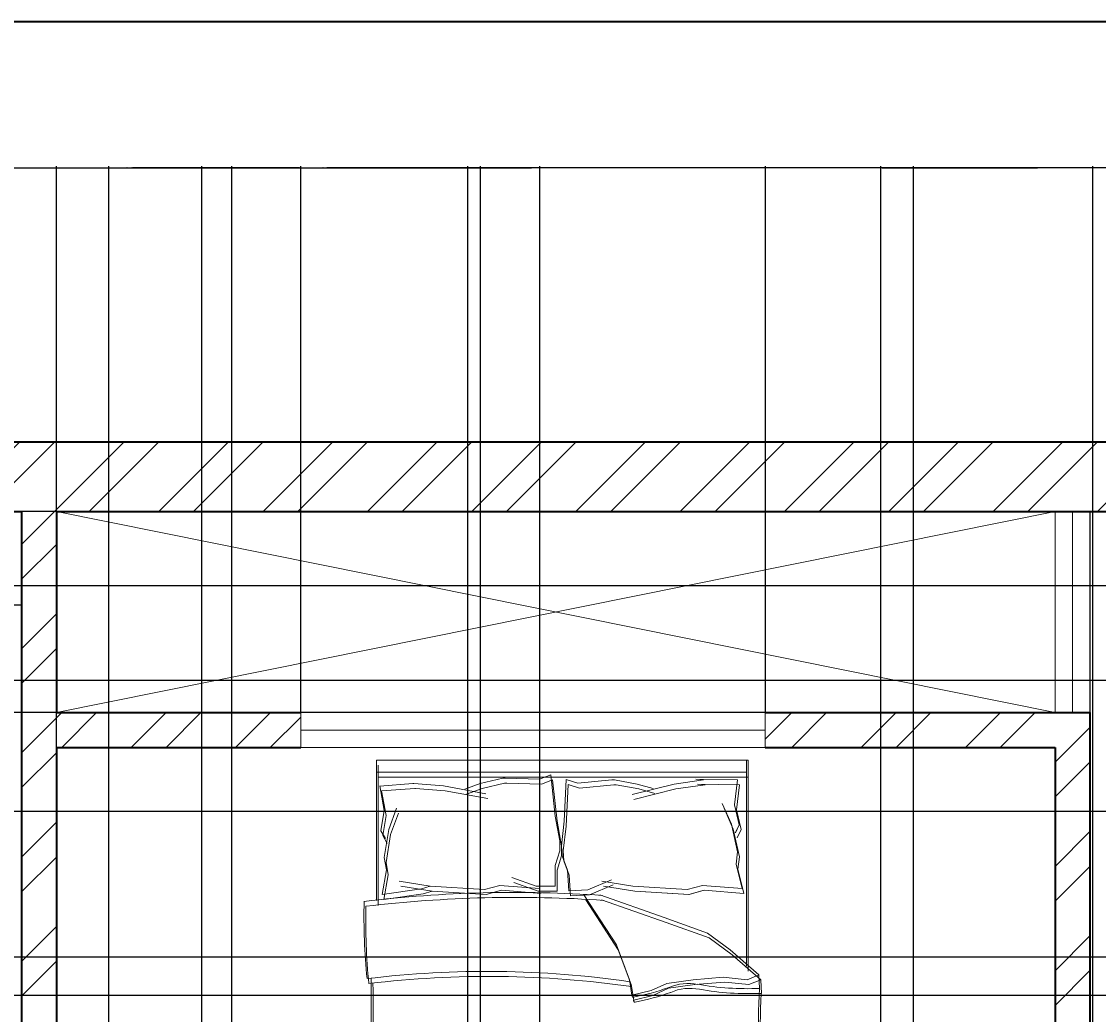
# Model space of a CAD drawing. Units: inches. Extents: x 2529 to 3014, y 1203 to 2262.
# Tile 12 of 13: x 2733 to 2872, y 2133 to 2262. Entities that reach past the tile are written whole.
import ezdxf

# ---------------------------------------------------------------- set-up
doc = ezdxf.new("R2010")
doc.units = ezdxf.units.IN
for name, color, linetype, lineweight in [('A-ANNO-DIMS', 2, 'Continuous', 18), ('A-ANNO-TTLB', 7, 'Continuous', 35), ('A-FLOR-CASE', 7, 'Continuous', 25), ('A-FLOR-OPEN', 61, 'Continuous', 13), ('A-FURN', 8, 'Continuous', 18), ('A-GLAZ', 191, 'Continuous', 18), ('A-WALL', 7, 'Continuous', 35), ('A-WALL-PATT', 143, 'Continuous', 13)]:
    doc.layers.add(name, color=color, linetype=linetype, lineweight=lineweight)
doc.styles.get("Standard").update_dxf_attribs({"font": 'arial.ttf'})
doc.dimstyles.get("Standard").update_dxf_attribs({"dimtxt": 0.18, "dimasz": 0.18, "dimexe": 0.18, "dimexo": 0.0625, "dimgap": 0.09, "dimtad": 0, "dimtih": 1, "dimtoh": 1, "dimdec": 4, "dimzin": 0, "dimdsep": 46, "dimtxsty": 'Standard', "dimcen": 0.09, "dimadec": 0, "dimazin": 0, "dimtfac": 1, "dimtdec": 4, "dimtofl": 0, "dimtmove": 0, "dimatfit": 3, "dimfxl": 1, "dimtolj": 1, "dimtzin": 0, "dimarcsym": 0})

# ---------------------------------------------------------------- blocks, each defined once
blk = doc.blocks.new('BED-DOUBLE')
for p, q in [((3.48, 63.33), (3.48, 81.44)), ((3.48, 63.33), (3.48, 81.44)), ((3.48, 81.44), (51.49, 81.44)), ((3.7, 62.69), (3.7, 80.8)), ((3.7, 62.69), (3.7, 80.8)), ((51.27, 81.44), (51.27, 54.83)), ((51.27, 81.44), (51.27, 54.83)), ((51.49, 81.44), (51.49, 80.8)), ((51.49, 80.8), (51.49, 54.19)), ((51.49, 80.8), (51.49, 54.19)), ((3.48, 79.91), (51.27, 79.91)), ((3.48, 79.91), (51.27, 79.91)), ((24.54, 78.99), (25.98, 79.57)), ((24.54, 78.99), (25.98, 79.57)), ((25.98, 79.57), (26.56, 74.22)), ((25.98, 79.57), (26.56, 74.22)), ((3.7, 79.27), (51.49, 79.27)), ((3.7, 79.27), (51.49, 79.27)), ((3.9, 78.11), (8.18, 78.43)), ((3.9, 78.11), (8.18, 78.43)), ((3.9, 78.13), (4.47, 74.95)), ((3.9, 78.13), (4.47, 74.95)), ((8.18, 78.43), (8.29, 78.42)), ((8.18, 78.43), (8.29, 78.42)), ((8.29, 78.42), (12.11, 78.13)), ((8.29, 78.42), (12.11, 78.13)), ((12.11, 78.13), (17.6, 77.12)), ((12.11, 78.13), (17.6, 77.12)), ((14.86, 77.69), (16.88, 78.42)), ((14.86, 77.69), (16.88, 78.42)), ((16.88, 78.42), (19.77, 79.14)), ((16.88, 78.42), (19.77, 79.14)), ((17.11, 77.78), (20, 78.5)), ((17.11, 77.78), (20, 78.5)), ((19.77, 79.14), (20.09, 79.14)), ((19.77, 79.14), (20.09, 79.14)), ((20, 78.5), (20.32, 78.5)), ((20, 78.5), (20.32, 78.5)), ((20.09, 79.14), (24.54, 78.99)), ((20.09, 79.14), (24.54, 78.99)), ((20.32, 78.5), (24.77, 78.36)), ((20.32, 78.5), (24.77, 78.36)), ((24.77, 78.36), (26.21, 78.93)), ((24.77, 78.36), (26.21, 78.93)), ((26.21, 78.93), (26.79, 73.58)), ((26.21, 78.93), (26.79, 73.58)), ((27.98, 78.95), (27.73, 73.58)), ((27.98, 78.95), (27.73, 73.58)), ((28.21, 78.31), (27.96, 72.94)), ((28.21, 78.31), (27.96, 72.94)), ((29.46, 78.46), (27.98, 78.95)), ((29.46, 78.46), (27.98, 78.95)), ((29.68, 77.83), (28.21, 78.31)), ((29.68, 77.83), (28.21, 78.31)), ((33.88, 78.89), (29.46, 78.46)), ((33.88, 78.89), (29.46, 78.46)), ((34.11, 78.25), (29.68, 77.83)), ((34.11, 78.25), (29.68, 77.83)), ((34.21, 78.91), (33.88, 78.89)), ((34.21, 78.91), (33.88, 78.89)), ((34.43, 78.27), (34.11, 78.25)), ((34.43, 78.27), (34.11, 78.25)), ((37.14, 78.37), (34.21, 78.91)), ((37.14, 78.37), (34.21, 78.91)), ((37.36, 77.73), (34.43, 78.27)), ((37.36, 77.73), (34.43, 78.27)), ((41.91, 78.37), (36.5, 77.02)), ((41.91, 78.37), (36.5, 77.02)), ((39.2, 77.77), (37.14, 78.37)), ((39.2, 77.77), (37.14, 78.37)), ((45.71, 78.9), (41.91, 78.37)), ((45.71, 78.9), (41.91, 78.37)), ((45.94, 78.26), (42.14, 77.73)), ((45.94, 78.26), (42.14, 77.73)), ((50.11, 78.89), (44.71, 78.98)), ((44.71, 78.98), (45.71, 78.9)), ((50.11, 78.89), (44.71, 78.98)), ((44.71, 78.98), (45.71, 78.9)), ((50.34, 78.25), (44.94, 78.34)), ((44.94, 78.34), (45.94, 78.26)), ((50.34, 78.25), (44.94, 78.34)), ((44.94, 78.34), (45.94, 78.26)), ((50.11, 78.89), (49.73, 75.68)), ((50.11, 78.89), (49.73, 75.68)), ((50.34, 78.25), (49.96, 75.04)), ((50.34, 78.25), (49.96, 75.04)), ((4.12, 77.49), (4.7, 74.31)), ((4.12, 77.49), (4.7, 74.31)), ((4.13, 77.47), (8.41, 77.8)), ((4.13, 77.47), (8.41, 77.8)), ((8.41, 77.8), (8.51, 77.78)), ((8.41, 77.8), (8.51, 77.78)), ((8.51, 77.78), (12.34, 77.49)), ((8.51, 77.78), (12.34, 77.49)), ((12.34, 77.49), (17.83, 76.48)), ((12.34, 77.49), (17.83, 76.48)), ((15.08, 77.05), (17.11, 77.78)), ((15.08, 77.05), (17.11, 77.78)), ((42.14, 77.73), (36.72, 76.38)), ((42.14, 77.73), (36.72, 76.38)), ((39.43, 77.13), (37.36, 77.73)), ((39.43, 77.13), (37.36, 77.73)), ((5.05, 72.49), (6.06, 75.24)), ((5.05, 72.49), (6.06, 75.24)), ((49.31, 73.19), (48.13, 75.87)), ((49.31, 73.19), (48.13, 75.87)), ((49.54, 72.55), (48.36, 75.23)), ((49.54, 72.55), (48.36, 75.23)), ((49.73, 75.68), (50.33, 73.11)), ((49.73, 75.68), (50.33, 73.11)), ((4.47, 74.95), (4.04, 72.34)), ((4.47, 74.95), (4.04, 72.34)), ((4.7, 74.31), (4.27, 71.7)), ((4.7, 74.31), (4.27, 71.7)), ((5.28, 71.85), (6.29, 74.6)), ((5.28, 71.85), (6.29, 74.6)), ((26.56, 74.22), (27.14, 71.04)), ((26.56, 74.22), (27.14, 71.04)), ((49.96, 75.04), (50.56, 72.47)), ((49.96, 75.04), (50.56, 72.47)), ((4.04, 72.34), (4.62, 71.33)), ((4.04, 72.34), (4.62, 71.33)), ((4.47, 68.87), (5.05, 72.49)), ((4.47, 68.87), (5.05, 72.49)), ((26.79, 73.58), (27.37, 70.4)), ((26.79, 73.58), (27.37, 70.4)), ((27.73, 73.58), (27.36, 70.37)), ((27.73, 73.58), (27.36, 70.37)), ((27.96, 72.94), (27.58, 69.73)), ((27.96, 72.94), (27.58, 69.73)), ((50.11, 69.61), (49.31, 73.19)), ((50.11, 69.61), (49.31, 73.19)), ((50.34, 68.98), (49.54, 72.55)), ((50.34, 68.98), (49.54, 72.55)), ((50.33, 73.11), (49.81, 72.06)), ((50.33, 73.11), (49.82, 72.06)), ((50.56, 72.47), (50.04, 71.42)), ((50.56, 72.47), (50.04, 71.42)), ((4.27, 71.7), (4.85, 70.69)), ((4.27, 71.7), (4.85, 70.69)), ((4.7, 68.23), (5.28, 71.85)), ((4.7, 68.23), (5.28, 71.85)), ((27.14, 71.04), (27.14, 69.74)), ((27.14, 71.04), (27.14, 69.74)), ((27.14, 69.74), (26.56, 67.86)), ((27.14, 69.74), (26.56, 67.86)), ((27.36, 70.37), (27.44, 69.07)), ((27.36, 70.37), (27.44, 69.07)), ((27.37, 70.4), (27.37, 69.1)), ((27.37, 70.4), (27.37, 69.1)), ((27.58, 69.73), (27.67, 68.43)), ((27.58, 69.73), (27.66, 68.43)), ((49.92, 68.01), (50.11, 69.61)), ((49.92, 68.01), (50.11, 69.61)), ((4.76, 67.28), (4.47, 68.87)), ((4.76, 67.28), (4.47, 68.87)), ((4.99, 66.64), (4.7, 68.23)), ((4.99, 66.64), (4.7, 68.23)), ((27.37, 69.1), (26.79, 67.22)), ((27.37, 69.1), (26.79, 67.22)), ((27.44, 69.07), (28.13, 67.23)), ((27.44, 69.07), (28.13, 67.23)), ((27.66, 68.43), (28.36, 66.59)), ((27.67, 68.43), (28.36, 66.59)), ((50.15, 67.37), (50.34, 68.98)), ((50.15, 67.37), (50.34, 68.98)), ((4.18, 64.1), (4.76, 67.28)), ((4.18, 64.1), (4.76, 67.28)), ((26.56, 67.86), (26.56, 65.18)), ((26.56, 67.86), (26.56, 65.18)), ((26.79, 67.22), (26.79, 64.54)), ((26.79, 67.22), (26.79, 64.54)), ((28.13, 67.23), (28.3, 64.55)), ((28.13, 67.23), (28.3, 64.55)), ((50.7, 64.87), (49.92, 68.01)), ((50.7, 64.87), (49.92, 68.01)), ((50.93, 64.23), (50.15, 67.37)), ((50.93, 64.23), (50.15, 67.37)), ((4.41, 63.46), (4.99, 66.64)), ((4.41, 63.46), (4.99, 66.64)), ((6.38, 65.81), (10.41, 65.15)), ((6.38, 65.81), (10.41, 65.15)), ((24.1, 65.18), (20.96, 66.27)), ((24.1, 65.18), (20.96, 66.27)), ((24.33, 64.54), (21.19, 65.63)), ((24.33, 64.54), (21.19, 65.63)), ((28.36, 66.59), (28.53, 63.91)), ((28.36, 66.59), (28.53, 63.91)), ((30.75, 64.7), (33.82, 65.99)), ((30.75, 64.7), (33.82, 65.99)), ((32.56, 65.81), (36.6, 65.15)), ((32.56, 65.81), (36.6, 65.15)), ((9.28, 64.83), (4.18, 64.1)), ((9.28, 64.83), (4.18, 64.1)), ((9.51, 64.19), (4.41, 63.46)), ((9.51, 64.19), (4.41, 63.46)), ((6.61, 65.18), (10.64, 64.51)), ((6.61, 65.18), (10.64, 64.51)), ((10.41, 65.15), (9.28, 64.83)), ((10.41, 65.15), (9.28, 64.83)), ((10.64, 64.51), (9.51, 64.19)), ((10.64, 64.51), (9.51, 64.19)), ((10.41, 65.15), (17.42, 64.72)), ((10.41, 65.15), (17.42, 64.72)), ((10.64, 64.51), (17.65, 64.08)), ((10.64, 64.51), (17.65, 64.08)), ((17.42, 64.72), (19.38, 65.27)), ((17.42, 64.72), (19.38, 65.27)), ((17.65, 64.08), (19.61, 64.64)), ((17.65, 64.08), (19.61, 64.64)), ((19.38, 65.27), (24.52, 64.87)), ((19.38, 65.27), (24.52, 64.87)), ((19.61, 64.64), (24.74, 64.23)), ((19.61, 64.64), (24.74, 64.23)), ((26.56, 65.18), (24.1, 65.18)), ((26.56, 65.18), (24.1, 65.18)), ((26.79, 64.54), (24.33, 64.54)), ((26.79, 64.54), (24.33, 64.54)), ((28.3, 64.55), (30.75, 64.7)), ((28.3, 64.55), (30.75, 64.7)), ((28.53, 63.91), (30.98, 64.06)), ((28.53, 63.91), (30.98, 64.06)), ((30.26, 64.06), (34.45, 57.57)), ((30.26, 64.06), (34.45, 57.57)), ((30.98, 64.06), (34.05, 65.35)), ((30.98, 64.06), (34.05, 65.35)), ((40.64, 61.13), (32.31, 64.06)), ((40.64, 61.13), (32.31, 64.06)), ((32.79, 65.18), (36.83, 64.51)), ((32.79, 65.18), (36.82, 64.51)), ((36.6, 65.15), (43.61, 64.72)), ((36.6, 65.15), (43.61, 64.72)), ((36.82, 64.51), (43.83, 64.08)), ((36.83, 64.51), (43.84, 64.08)), ((43.61, 64.72), (45.57, 65.27)), ((43.61, 64.72), (45.57, 65.27)), ((43.83, 64.08), (45.8, 64.64)), ((43.84, 64.08), (45.8, 64.64)), ((45.57, 65.27), (50.7, 64.87)), ((45.57, 65.27), (50.7, 64.87)), ((45.8, 64.64), (50.93, 64.23)), ((45.8, 64.64), (50.93, 64.23)), ((30.49, 63.42), (34.68, 56.93)), ((30.49, 63.42), (34.68, 56.93)), ((40.87, 60.49), (32.53, 63.42)), ((40.87, 60.49), (32.54, 63.42)), ((46.22, 59.11), (40.64, 61.13)), ((46.22, 59.11), (40.64, 61.13)), ((46.45, 58.48), (40.87, 60.49)), ((46.45, 58.48), (40.87, 60.49)), ((49.16, 56.95), (46.22, 59.11)), ((49.16, 56.95), (46.22, 59.11)), ((49.39, 56.31), (46.45, 58.48)), ((49.39, 56.31), (46.45, 58.48)), ((34.45, 57.57), (36.15, 53.08)), ((34.45, 57.57), (36.15, 53.08)), ((34.68, 56.93), (36.38, 52.44)), ((34.68, 56.93), (36.38, 52.44)), ((52.87, 53.7), (49.16, 56.95)), ((52.87, 53.7), (49.16, 56.95)), ((53.1, 53.06), (49.39, 56.31)), ((53.1, 53.06), (49.39, 56.31)), ((36.15, 53.08), (36.46, 51.07)), ((36.15, 53.08), (36.46, 51.07)), ((40.95, 52.61), (44.36, 53.08)), ((40.95, 52.61), (44.36, 53.08)), ((44.36, 53.08), (48.23, 53.39)), ((44.36, 53.08), (48.23, 53.39)), ((48.23, 53.39), (51.33, 53.08)), ((48.23, 53.39), (51.33, 53.08)), ((51.33, 53.08), (52.87, 53.7)), ((51.33, 53.08), (52.87, 53.7)), ((51.56, 52.44), (53.1, 53.06)), ((51.56, 52.44), (53.1, 53.06)), ((52.95, 51.95), (52.87, 53.7, 3.87)), ((52.95, 51.95), (52.87, 53.7, 3.87)), ((53.18, 51.31), (53.1, 53.06, 3.87)), ((53.18, 51.31), (53.1, 53.06, 3.87)), ((36.38, 52.44), (36.69, 50.43)), ((36.38, 52.44), (36.69, 50.43)), ((36.46, 51.07), (38.94, 51.69)), ((36.46, 51.07), (38.94, 51.69)), ((38.94, 51.69), (40.95, 52.61)), ((38.94, 51.69), (40.95, 52.61)), ((39.17, 51.05), (41.18, 51.97)), ((39.17, 51.05), (41.18, 51.97)), ((41.18, 51.97), (44.59, 52.44)), ((41.18, 51.97), (44.59, 52.44)), ((44.59, 52.44), (48.46, 52.75)), ((44.59, 52.44), (48.46, 52.75)), ((48.46, 52.75), (51.56, 52.44)), ((48.46, 52.75), (51.56, 52.44)), ((36.69, 50.43), (39.17, 51.05)), ((36.69, 50.43), (39.17, 51.05)), ((15.06, 2.2), (39.68, 2.2)), ((15.06, 2.2), (39.68, 2.2)), ((15.29, 1.56), (39.91, 1.56)), ((15.29, 1.56), (39.91, 1.56))]:
    blk.add_line(p, q)
for centre, radius, start, end in [((21.36, -100.61), 164.97, 86.0865, 96.7821), ((21.36, -100.61), 164.97, 86.0865, 96.7821), ((85.16, 61.35), 83.31, 178.7218, 185.604), ((85.16, 61.35), 83.31, 178.7218, 185.604), ((21.59, -101.25), 164.97, 86.0865, 96.7821), ((21.59, -101.25), 164.97, 86.0865, 96.7821), ((85.39, 60.71), 83.31, 178.7218, 185.604), ((85.39, 60.71), 83.31, 178.7218, 185.604), ((17.76, -74.87), 129.02, 81.7845, 96.9006), ((17.76, -74.87), 129.02, 81.7845, 96.9006), ((17.98, -75.51), 129.02, 81.7845, 96.9006), ((17.98, -75.51), 129.02, 81.7845, 96.9006), ((-167.31, 50.27), 170.11, 358.4762, 1.0082), ((-167.31, 50.27), 170.11, 358.4762, 1.0082), ((-167.08, 49.63), 170.11, 358.4762, 1.0082), ((-167.08, 49.63), 170.11, 358.4762, 1.0082), ((31.15, 79.96), 29.65, 280.6617, 289.8806), ((31.15, 79.96), 29.65, 280.6617, 289.8806), ((43.74, 46.38), 6.22, 78.6608, 113.7384), ((43.74, 46.38), 6.22, 78.6608, 113.7384), ((43.97, 45.74), 6.22, 78.6608, 113.7384), ((43.97, 45.74), 6.22, 78.6608, 113.7384), ((51.33, 88.1), 36.18, 259.8763, 272.5657), ((51.33, 88.1), 36.18, 259.8763, 272.5657), ((51.56, 87.46), 36.18, 259.8763, 272.5657), ((51.56, 87.46), 36.18, 259.8763, 272.5657), ((182.27, 45.13), 129.5, 176.9791, 183.8365), ((182.27, 45.13), 129.5, 176.9791, 183.8365), ((36.64, 51), 0.185, 160.2464, 271.1377), ((36.64, 51), 0.185, 160.2464, 271.1377), ((36.87, 50.36), 0.185, 160.2464, 271.1377), ((36.86, 50.36), 0.185, 160.2464, 271.1377), ((31.38, 79.32), 29.65, 280.6617, 289.8806), ((31.38, 79.32), 29.65, 280.6617, 289.8806), ((182.49, 44.49), 129.5, 176.9791, 183.8365), ((182.49, 44.49), 129.5, 176.9791, 183.8365), ((484.82, 30.83), 482.31, 178.2277, 181.7185), ((484.82, 30.83), 482.31, 178.2277, 181.7185), ((485.05, 30.19), 482.31, 178.2277, 181.7185), ((485.05, 30.19), 482.31, 178.2277, 181.7185), ((-4508.74, 13.62), 4561.86, 0.00217, 0.28689), ((-4508.74, 13.62), 4561.86, 0.00217, 0.28689), ((-4508.51, 12.98), 4561.86, 0.00217, 0.28689), ((-4508.51, 12.98), 4561.86, 0.00217, 0.28689), ((-26.9, 16.93), 29.63, 346.0648, 358.9113), ((-26.9, 16.93), 29.63, 346.0648, 358.9113), ((-26.67, 16.29), 29.63, 346.0648, 358.9113), ((-26.67, 16.29), 29.63, 346.0648, 358.9113), ((76.16, 12.78), 23.07, 177.4714, 206.4681), ((76.16, 12.78), 23.07, 177.4714, 206.4681), ((76.39, 12.14), 23.07, 177.4714, 206.4681), ((76.39, 12.14), 23.07, 177.4714, 206.4681), ((-21.66, 11.17), 23.56, 337.9751, 356.652), ((-21.66, 11.17), 23.56, 337.9751, 356.652), ((-21.43, 10.53), 23.56, 337.9751, 356.652), ((-21.43, 10.53), 23.56, 337.9751, 356.652), ((-17.22, 105.16), 106.46, 283.3832, 287.7053), ((-17.22, 105.16), 106.46, 283.3832, 287.7053), ((-16.99, 104.52), 106.46, 283.3832, 287.7053), ((-16.99, 104.52), 106.46, 283.3832, 287.7053), ((1.09, 1.73), 1.09, 146.1736, 293.4781), ((1.09, 1.73), 1.09, 146.1736, 293.4781), ((1.32, 1.09), 1.09, 146.1736, 293.4781), ((1.32, 1.09), 1.09, 146.1736, 293.4781), ((21.43, -119.39), 121.76, 92.9958, 99.4091), ((21.43, -119.39), 121.76, 92.9958, 99.4091), ((21.66, -120.03), 121.76, 92.9958, 99.4091), ((21.66, -120.03), 121.76, 92.9958, 99.4091), ((41.15, -130.83), 133.04, 84.4998, 90.6351), ((41.15, -130.83), 133.04, 84.4998, 90.6351), ((41.38, -131.47), 133.04, 84.4998, 90.6351), ((41.38, -131.47), 133.04, 84.4998, 90.6351), ((54.41, 2.57), 1.1, 242.6588, 356.02), ((54.41, 2.57), 1.1, 242.6588, 356.02), ((54.64, 1.93), 1.1, 242.6588, 356.02), ((54.64, 1.93), 1.1, 242.6588, 356.02)]:
    blk.add_arc(centre, radius, start, end)
blk = doc.blocks.new('*D16')
at = {"layer": 'A-ANNO-DIMS', "color": 0, "lineweight": -2, "transparency": 16777216}
for p, q in [((2577.06, 2207.57), (2577.06, 2243.11)), ((2577.24, 2242.93), (2774.27, 2242.93)), ((2971.88, 2242.93), (2774.84, 2242.93)), ((2972.06, 2207.57), (2972.06, 2243.11))]:
    blk.add_line(p, q, dxfattribs=at)
at = {"layer": 'A-ANNO-DIMS', "color": 0, "transparency": 16777216}
for points in [[(2577.24, 2242.96), (2577.24, 2242.9), (2577.06, 2242.93)], [(2971.88, 2242.96), (2971.88, 2242.9), (2972.06, 2242.93)]]:
    blk.add_solid(points, dxfattribs=at)
at = {"layer": 'Defpoints', "color": 0, "transparency": 16777216}
for p in [(2972.06, 2242.93), (2577.06, 2207.5), (2972.06, 2207.5)]:
    blk.add_point(p, dxfattribs=at)
at = {"layer": 'A-ANNO-DIMS', "color": 0, "transparency": 16777216, "insert": (2774.56, 2242.93), "char_height": 0.18, "attachment_point": 5}
blk.add_mtext('\\A1;395', dxfattribs=at)
blk = doc.blocks.new('*D36')
at = {"layer": 'A-ANNO-DIMS', "color": 0, "lineweight": -2, "transparency": 16777216}
for p, q in [((2737.56, 1582.57), (2737.56, 2243.11)), ((2737.74, 2242.93), (2746.49, 2242.93)), ((2756.15, 2242.93), (2747.4, 2242.93)), ((2756.33, 1582.57), (2756.33, 2243.11))]:
    blk.add_line(p, q, dxfattribs=at)
at = {"layer": 'A-ANNO-DIMS', "color": 0, "transparency": 16777216}
for points in [[(2737.74, 2242.96), (2737.74, 2242.9), (2737.56, 2242.93)], [(2756.15, 2242.96), (2756.15, 2242.9), (2756.33, 2242.93)]]:
    blk.add_solid(points, dxfattribs=at)
at = {"layer": 'Defpoints', "color": 0, "transparency": 16777216}
for p in [(2756.33, 2242.93), (2737.56, 1582.5), (2756.33, 1582.5)]:
    blk.add_point(p, dxfattribs=at)
at = {"layer": 'A-ANNO-DIMS', "color": 0, "transparency": 16777216, "insert": (2746.94, 2242.93), "char_height": 0.18, "attachment_point": 5}
blk.add_mtext('\\A1;18.778', dxfattribs=at)
blk = doc.blocks.new('*D37')
at = {"layer": 'A-ANNO-DIMS', "color": 0, "lineweight": -2, "transparency": 16777216}
for p, q in [((2756.33, 1582.57), (2756.33, 2243.11)), ((2756.51, 2242.93), (2774.11, 2242.93)), ((2792.15, 2242.93), (2774.55, 2242.93)), ((2792.33, 1582.57), (2792.33, 2243.11))]:
    blk.add_line(p, q, dxfattribs=at)
at = {"layer": 'A-ANNO-DIMS', "color": 0, "transparency": 16777216}
for points in [[(2756.51, 2242.96), (2756.51, 2242.9), (2756.33, 2242.93)], [(2792.15, 2242.96), (2792.15, 2242.9), (2792.33, 2242.93)]]:
    blk.add_solid(points, dxfattribs=at)
at = {"layer": 'Defpoints', "color": 0, "transparency": 16777216}
for p in [(2792.33, 2242.93), (2756.33, 1582.5), (2792.33, 1582.5)]:
    blk.add_point(p, dxfattribs=at)
at = {"layer": 'A-ANNO-DIMS', "color": 0, "transparency": 16777216, "insert": (2774.33, 2242.93), "char_height": 0.18, "attachment_point": 5}
blk.add_mtext('\\A1;36', dxfattribs=at)
blk = doc.blocks.new('*D38')
at = {"layer": 'A-ANNO-DIMS', "color": 0, "lineweight": -2, "transparency": 16777216}
for p, q in [((2844.06, 1582.57), (2844.06, 2243.11)), ((2844.24, 2242.93), (2857.35, 2242.93)), ((2871.26, 2242.93), (2858.14, 2242.93)), ((2871.44, 1582.57), (2871.44, 2243.11))]:
    blk.add_line(p, q, dxfattribs=at)
at = {"layer": 'A-ANNO-DIMS', "color": 0, "transparency": 16777216}
for points in [[(2844.24, 2242.96), (2844.24, 2242.9), (2844.06, 2242.93)], [(2871.26, 2242.96), (2871.26, 2242.9), (2871.44, 2242.93)]]:
    blk.add_solid(points, dxfattribs=at)
at = {"layer": 'Defpoints', "color": 0, "transparency": 16777216}
for p in [(2871.44, 2242.93), (2844.06, 1582.5), (2871.44, 1582.5)]:
    blk.add_point(p, dxfattribs=at)
at = {"layer": 'A-ANNO-DIMS', "color": 0, "transparency": 16777216, "insert": (2857.75, 2242.93), "char_height": 0.18, "attachment_point": 5}
blk.add_mtext('\\A1;27.39', dxfattribs=at)
blk = doc.blocks.new('*D39')
at = {"layer": 'A-ANNO-DIMS', "color": 0, "lineweight": -2, "transparency": 16777216}
for p, q in [((2848.27, 1734.07), (2848.27, 2243.11)), ((2848.45, 2242.93), (2864.3, 2242.93)), ((2881.08, 2242.93), (2865.23, 2242.93)), ((2881.26, 1734.07), (2881.26, 2243.11))]:
    blk.add_line(p, q, dxfattribs=at)
at = {"layer": 'A-ANNO-DIMS', "color": 0, "transparency": 16777216}
for points in [[(2848.45, 2242.96), (2848.45, 2242.9), (2848.27, 2242.93)], [(2881.08, 2242.96), (2881.08, 2242.9), (2881.26, 2242.93)]]:
    blk.add_solid(points, dxfattribs=at)
at = {"layer": 'Defpoints', "color": 0, "transparency": 16777216}
for p in [(2881.26, 2242.93), (2848.27, 1734), (2881.26, 1734)]:
    blk.add_point(p, dxfattribs=at)
at = {"layer": 'A-ANNO-DIMS', "color": 0, "transparency": 16777216, "insert": (2864.76, 2242.93), "char_height": 0.18, "attachment_point": 5}
blk.add_mtext('\\A1;32.994', dxfattribs=at)
blk = doc.blocks.new('*D40')
at = {"layer": 'A-ANNO-DIMS', "color": 0, "lineweight": -2, "transparency": 16777216}
for p, q in [((2744.32, 1738.57), (2744.32, 2243.11)), ((2744.5, 2242.93), (2771.84, 2242.93)), ((2799.84, 2242.93), (2772.49, 2242.93)), ((2800.02, 1738.57), (2800.02, 2243.11))]:
    blk.add_line(p, q, dxfattribs=at)
at = {"layer": 'A-ANNO-DIMS', "color": 0, "transparency": 16777216}
for points in [[(2744.5, 2242.96), (2744.5, 2242.9), (2744.32, 2242.93)], [(2799.84, 2242.96), (2799.84, 2242.9), (2800.02, 2242.93)]]:
    blk.add_solid(points, dxfattribs=at)
at = {"layer": 'Defpoints', "color": 0, "transparency": 16777216}
for p in [(2800.02, 2242.93), (2744.32, 1738.5), (2800.02, 1738.5)]:
    blk.add_point(p, dxfattribs=at)
at = {"layer": 'A-ANNO-DIMS', "color": 0, "transparency": 16777216, "insert": (2772.17, 2242.93), "char_height": 0.18, "attachment_point": 5}
blk.add_mtext('\\A1;55.7', dxfattribs=at)
blk = doc.blocks.new('*D46')
at = {"layer": 'A-ANNO-DIMS', "color": 0, "lineweight": -2, "transparency": 16777216}
for p, q in [((2613.12, 2188.94), (3007.66, 2188.94)), ((3007.48, 2188.76), (3007.48, 2165.12)), ((3007.48, 2141.12), (3007.48, 2164.75)), ((2613.12, 2140.94), (3007.66, 2140.94))]:
    blk.add_line(p, q, dxfattribs=at)
at = {"layer": 'A-ANNO-DIMS', "color": 0, "transparency": 16777216}
for points in [[(3007.45, 2188.76), (3007.51, 2188.76), (3007.48, 2188.94)], [(3007.45, 2141.12), (3007.51, 2141.12), (3007.48, 2140.94)]]:
    blk.add_solid(points, dxfattribs=at)
at = {"layer": 'Defpoints', "color": 0, "transparency": 16777216}
for p in [(2613.06, 2188.94), (3007.48, 2188.94), (2613.06, 2140.94)]:
    blk.add_point(p, dxfattribs=at)
at = {"layer": 'A-ANNO-DIMS', "color": 0, "transparency": 16777216, "insert": (3007.48, 2164.94), "char_height": 0.18, "attachment_point": 5}
blk.add_mtext('\\A1;48', dxfattribs=at)
blk = doc.blocks.new('*D54')
at = {"layer": 'A-ANNO-DIMS', "color": 0, "lineweight": -2, "transparency": 16777216}
for p, q in [((2866.49, 2198.5), (2541.45, 2198.5)), ((2541.63, 2198.32), (2541.63, 2185.69)), ((2541.63, 2172.68), (2541.63, 2185.32)), ((2866.49, 2172.5), (2541.45, 2172.5))]:
    blk.add_line(p, q, dxfattribs=at)
at = {"layer": 'A-ANNO-DIMS', "color": 0, "transparency": 16777216}
for points in [[(2541.6, 2198.32), (2541.66, 2198.32), (2541.63, 2198.5)], [(2541.6, 2172.68), (2541.66, 2172.68), (2541.63, 2172.5)]]:
    blk.add_solid(points, dxfattribs=at)
at = {"layer": 'Defpoints', "color": 0, "transparency": 16777216}
for p in [(2541.63, 2198.5), (2866.56, 2198.5), (2866.56, 2172.5)]:
    blk.add_point(p, dxfattribs=at)
at = {"layer": 'A-ANNO-DIMS', "color": 0, "transparency": 16777216, "insert": (2541.63, 2185.5), "char_height": 0.18, "attachment_point": 5}
blk.add_mtext('\\A1;26', dxfattribs=at)
blk = doc.blocks.new('*D55')
at = {"layer": 'A-ANNO-DIMS', "color": 0, "lineweight": -2, "transparency": 16777216}
for p, q in [((2737.56, 2172.57), (2737.56, 2243.11)), ((2737.74, 2242.93), (2752.95, 2242.93)), ((2768.95, 2242.93), (2753.73, 2242.93)), ((2769.13, 2172.57), (2769.13, 2243.11))]:
    blk.add_line(p, q, dxfattribs=at)
at = {"layer": 'A-ANNO-DIMS', "color": 0, "transparency": 16777216}
for points in [[(2737.74, 2242.96), (2737.74, 2242.9), (2737.56, 2242.93)], [(2768.95, 2242.96), (2768.95, 2242.9), (2769.13, 2242.93)]]:
    blk.add_solid(points, dxfattribs=at)
at = {"layer": 'Defpoints', "color": 0, "transparency": 16777216}
for p in [(2769.13, 2242.93), (2737.56, 2172.5), (2769.13, 2172.5)]:
    blk.add_point(p, dxfattribs=at)
at = {"layer": 'A-ANNO-DIMS', "color": 0, "transparency": 16777216, "insert": (2753.34, 2242.93), "char_height": 0.18, "attachment_point": 5}
blk.add_mtext('\\A1;31.57', dxfattribs=at)
blk = doc.blocks.new('*D56')
at = {"layer": 'A-ANNO-DIMS', "color": 0, "lineweight": -2, "transparency": 16777216}
for p, q in [((2769.13, 2172.57), (2769.13, 2243.11)), ((2769.31, 2242.93), (2798.91, 2242.93)), ((2828.95, 2242.93), (2799.35, 2242.93)), ((2829.13, 2172.57), (2829.13, 2243.11))]:
    blk.add_line(p, q, dxfattribs=at)
at = {"layer": 'A-ANNO-DIMS', "color": 0, "transparency": 16777216}
for points in [[(2769.31, 2242.96), (2769.31, 2242.9), (2769.13, 2242.93)], [(2828.95, 2242.96), (2828.95, 2242.9), (2829.13, 2242.93)]]:
    blk.add_solid(points, dxfattribs=at)
at = {"layer": 'Defpoints', "color": 0, "transparency": 16777216}
for p in [(2829.13, 2242.93), (2769.13, 2172.5), (2829.13, 2172.5)]:
    blk.add_point(p, dxfattribs=at)
at = {"layer": 'A-ANNO-DIMS', "color": 0, "transparency": 16777216, "insert": (2799.13, 2242.93), "char_height": 0.18, "attachment_point": 5}
blk.add_mtext('\\A1;60', dxfattribs=at)
blk = doc.blocks.new('*D57')
at = {"layer": 'A-ANNO-DIMS', "color": 0, "lineweight": -2, "transparency": 16777216}
for p, q in [((2871.06, 2198.44), (2871.06, 1483.77)), ((2893.92, 2198.44), (2893.92, 1483.77)), ((2871.24, 1483.95), (2882.02, 1483.95)), ((2893.74, 1483.95), (2882.95, 1483.95))]:
    blk.add_line(p, q, dxfattribs=at)
at = {"layer": 'A-ANNO-DIMS', "color": 0, "transparency": 16777216}
for points in [[(2871.24, 1483.98), (2871.24, 1483.92), (2871.06, 1483.95)], [(2893.74, 1483.98), (2893.74, 1483.92), (2893.92, 1483.95)]]:
    blk.add_solid(points, dxfattribs=at)
at = {"layer": 'Defpoints', "color": 0, "transparency": 16777216}
for p in [(2871.06, 2198.5), (2893.92, 2198.5), (2893.92, 1483.95)]:
    blk.add_point(p, dxfattribs=at)
at = {"layer": 'A-ANNO-DIMS', "color": 0, "transparency": 16777216, "insert": (2882.49, 1483.95), "char_height": 0.18, "attachment_point": 5}
blk.add_mtext('\\A1;22.866', dxfattribs=at)
blk = doc.blocks.new('*D72')
at = {"layer": 'A-ANNO-DIMS', "color": 0, "lineweight": -2, "transparency": 16777216}
for p, q in [((2631.64, 2176.7), (3007.66, 2176.7)), ((3007.48, 2176.52), (3007.48, 2168.41)), ((3007.48, 2159.93), (3007.48, 2168.04)), ((2631.64, 2159.75), (3007.66, 2159.75))]:
    blk.add_line(p, q, dxfattribs=at)
at = {"layer": 'A-ANNO-DIMS', "color": 0, "transparency": 16777216}
for points in [[(3007.45, 2176.52), (3007.51, 2176.52), (3007.48, 2176.7)], [(3007.45, 2159.93), (3007.51, 2159.93), (3007.48, 2159.75)]]:
    blk.add_solid(points, dxfattribs=at)
at = {"layer": 'Defpoints', "color": 0, "transparency": 16777216}
for p in [(2631.58, 2176.7), (3007.48, 2176.7), (2631.58, 2159.75)]:
    blk.add_point(p, dxfattribs=at)
at = {"layer": 'A-ANNO-DIMS', "color": 0, "transparency": 16777216, "insert": (3007.48, 2168.22), "char_height": 0.18, "attachment_point": 5}
blk.add_mtext('\\A1;16.957', dxfattribs=at)
blk = doc.blocks.new('*D73')
at = {"layer": 'A-ANNO-DIMS', "color": 0, "lineweight": -2, "transparency": 16777216}
for p, q in [((2631.64, 2159.75), (3007.66, 2159.75)), ((3007.48, 2159.57), (3007.48, 2148.04)), ((3007.48, 2136.16), (3007.48, 2147.68)), ((2634.12, 2135.98), (3007.66, 2135.98))]:
    blk.add_line(p, q, dxfattribs=at)
at = {"layer": 'A-ANNO-DIMS', "color": 0, "transparency": 16777216}
for points in [[(3007.45, 2159.57), (3007.51, 2159.57), (3007.48, 2159.75)], [(3007.45, 2136.16), (3007.51, 2136.16), (3007.48, 2135.98)]]:
    blk.add_solid(points, dxfattribs=at)
at = {"layer": 'Defpoints', "color": 0, "transparency": 16777216}
for p in [(2631.58, 2159.75), (2634.06, 2135.98), (3007.48, 2135.98)]:
    blk.add_point(p, dxfattribs=at)
at = {"layer": 'A-ANNO-DIMS', "color": 0, "transparency": 16777216, "insert": (3007.48, 2147.86), "char_height": 0.18, "attachment_point": 5}
blk.add_mtext('\\A1;23.77', dxfattribs=at)
blk = doc.blocks.new('*D78')
at = {"layer": 'A-ANNO-DIMS', "color": 0, "lineweight": -2, "transparency": 16777216}
for p, q in [((2760.22, 1599.16), (2760.22, 2243.11)), ((2760.4, 2242.93), (2775.15, 2242.93)), ((2790.54, 2242.93), (2775.8, 2242.93)), ((2790.72, 1599.16), (2790.72, 2243.11))]:
    blk.add_line(p, q, dxfattribs=at)
at = {"layer": 'A-ANNO-DIMS', "color": 0, "transparency": 16777216}
for points in [[(2760.4, 2242.96), (2760.4, 2242.9), (2760.22, 2242.93)], [(2790.54, 2242.96), (2790.54, 2242.9), (2790.72, 2242.93)]]:
    blk.add_solid(points, dxfattribs=at)
at = {"layer": 'Defpoints', "color": 0, "transparency": 16777216}
for p in [(2790.72, 2242.93), (2760.22, 1599.1), (2790.72, 1599.1)]:
    blk.add_point(p, dxfattribs=at)
at = {"layer": 'A-ANNO-DIMS', "color": 0, "transparency": 16777216, "insert": (2775.47, 2242.93), "char_height": 0.18, "attachment_point": 5}
blk.add_mtext('\\A1;30.5', dxfattribs=at)

msp = doc.modelspace()

# ---------------------------------------------------------------- hatches: boundary and pattern name
at = {"layer": 'A-WALL-PATT'}
h = msp.add_hatch(dxfattribs=at)
h.set_pattern_fill('ANSI32', color=256)
h.paths.add_polyline_path([(2686.5554, 2106.5032), (2622.0554, 2106.5032), (2622.0554, 2109.2964), (2617.4223, 2109.2964), (2613.0554, 2109.2964), (2613.0554, 2106.5032), (2577.0554, 2106.5032), (2577.0554, 2092.6918), (2586.0554, 2092.6918), (2586.0554, 2102.0032), (2682.0554, 2102.0032), (2682.0554, 2099.9833), (2686.5554, 2099.9833), (2686.5554, 2102.0032)])
h.paths.add_polyline_path([(2695.2249, 2054.0032), (2686.5554, 2054.0032), (2686.5554, 2080.2316), (2684.3054, 2080.2316), (2682.0554, 2080.2316), (2682.0554, 2054.0032), (2586.0554, 2054.0032), (2586.0554, 2068.6918), (2577.0554, 2068.6918), (2577.0554, 2019.1229), (2586.0554, 2019.1229), (2586.0554, 2049.5032), (2695.2249, 2049.5032)])
h.paths.add_polyline_path([(2737.5554, 2049.5032), (2866.5554, 2049.5032), (2866.5554, 2045.0233), (2871.0554, 2045.0233), (2871.0554, 2049.5032), (2871.0554, 2172.5032), (2866.5554, 2172.5032), (2829.1265, 2172.5032), (2829.1265, 2168.0032), (2866.5554, 2168.0032), (2866.5554, 2054.0032), (2737.5554, 2054.0032), (2737.5554, 2056.4892), (2735.3054, 2056.4892), (2733.0554, 2056.4892), (2733.0554, 2049.5032), (2733.0554, 1917.5032), (2733.0554, 1913.0032), (2871.0554, 1913.0032), (2871.0554, 1924.9149), (2868.8054, 1924.9149), (2866.5554, 1924.9149), (2866.5554, 1917.5032), (2737.5554, 1917.5032)], flags=17)
h.paths.add_polyline_path([(2972.0554, 2207.5032), (2613.0554, 2207.5032), (2613.0554, 2205.5032), (2613.0554, 2188.9366), (2622.0554, 2188.9366), (2622.0554, 2198.5032), (2733.0554, 2198.5032), (2733.0554, 2084.8053), (2735.3054, 2084.8053), (2737.5554, 2084.8053), (2737.5554, 2168.0032), (2769.1265, 2168.0032), (2769.1265, 2170.2532), (2769.1265, 2172.5032), (2737.5554, 2172.5032), (2737.5554, 2198.5032), (2963.0554, 2198.5032), (2963.0554, 2093.5032), (2912.0586, 2093.5032), (2912.0586, 2089.0032), (2918.5554, 2089.0032), (2918.5554, 2031.8749), (2923.0554, 2031.8749), (2923.0554, 2089.0032), (2963.0554, 2089.0032), (2963.0554, 2010.0032), (2923.0554, 2010.0032), (2923.0554, 2011.9417), (2918.5554, 2011.9417), (2918.5554, 2003.1338), (2923.0554, 2003.1338), (2923.0554, 2005.5032), (2963.0554, 2005.5032), (2963.0554, 1917.5032), (2963.0554, 1691.0776), (2972.0554, 1691.0776), (2972.0554, 1917.5032)])
h.paths.add_polyline_path([(2963.0554, 1945.5032), (2923.0554, 1945.5032), (2923.0554, 1983.0571), (2920.8054, 1983.0571), (2918.5554, 1983.0571), (2918.5554, 1941.0032), (2963.0554, 1941.0032)], flags=17)
h.paths.add_polyline_path([(2930.3679, 1788.7532), (2930.3679, 1791.0032), (2894.8637, 1791.0032), (2894.8637, 1786.5032), (2900.5554, 1786.5032), (2900.5554, 1784.6931), (2905.0554, 1784.6931), (2905.0554, 1786.5032), (2930.3679, 1786.5032)], flags=17)
h.paths.add_polyline_path([(2963.0554, 1791.0032), (2954.3679, 1791.0032), (2954.3679, 1786.5032), (2963.0554, 1786.5032)], flags=17)
h.paths.add_polyline_path([(2871.0554, 1853.0032), (2919.0554, 1853.0032), (2919.0554, 1847.0972), (2923.5554, 1847.0972), (2923.5554, 1853.0032), (2923.5554, 1857.5032), (2871.0554, 1857.5032), (2871.0554, 1871.7024), (2866.5554, 1871.7024), (2866.5554, 1791.0032), (2737.5554, 1791.0032), (2737.5554, 1806.6712), (2735.3054, 1806.6712), (2733.0554, 1806.6712), (2733.0554, 1791.0032), (2733.0554, 1786.5032), (2733.0554, 1780.6235), (2737.5554, 1780.6235), (2737.5554, 1786.5032), (2872.8745, 1786.5032), (2872.8745, 1788.7532), (2872.8745, 1791.0032), (2871.0554, 1791.0032)], flags=17)
h.paths.add_polyline_path([(2844.0554, 1734.0032), (2848.2652, 1734.0032), (2848.2652, 1738.5032), (2800.0167, 1738.5032), (2800.0167, 1734.0032), (2839.5554, 1734.0032), (2839.5554, 1582.5032), (2792.3334, 1582.5032), (2792.3334, 1573.5032), (2871.4433, 1573.5032), (2871.4433, 1578.0032), (2871.4433, 1582.5032), (2844.0554, 1582.5032)])
h.paths.add_polyline_path([(2972.0554, 1631.0776), (2963.0554, 1631.0776), (2963.0554, 1582.5032), (2931.4433, 1582.5032), (2931.4433, 1573.5032), (2972.0554, 1573.5032)])
h.paths.add_polyline_path([(2756.3334, 1582.5032), (2737.5554, 1582.5032), (2737.5554, 1734.0032), (2744.3201, 1734.0032), (2744.3201, 1738.5032), (2737.5554, 1738.5032), (2737.5554, 1746.0094), (2733.0554, 1746.0094), (2733.0554, 1738.5032), (2733.0554, 1612.5032), (2728.2475, 1612.5032), (2728.2475, 1603.5032), (2733.0554, 1603.5032), (2733.0554, 1582.5032), (2733.0554, 1573.5032), (2756.3334, 1573.5032), (2756.3334, 1578.0032)])
h.paths.add_polyline_path([(2695.7662, 1612.5032), (2658.4771, 1612.5032), (2658.4771, 1603.5032), (2695.7662, 1603.5032), (2695.7662, 1608.0032)])
h.paths.add_polyline_path([(2586.0554, 1686.9483), (2577.0554, 1686.9483), (2577.0554, 1603.5032), (2598.4771, 1603.5032), (2598.4771, 1608.0032), (2598.4771, 1612.5032), (2586.0554, 1612.5032)])
h.paths.add_polyline_path([(2683.2727, 1791.0032), (2586.0554, 1791.0032), (2586.0554, 1815.6736), (2581.5554, 1815.6736), (2577.0554, 1815.6736), (2577.0554, 1746.9483), (2586.0554, 1746.9483), (2586.0554, 1786.5032), (2683.2727, 1786.5032)])
h.paths.add_polyline_path([(2586.0554, 1959.1229), (2577.0554, 1959.1229), (2577.0554, 1875.6736), (2586.0554, 1875.6736), (2586.0554, 1913.0032), (2683.2727, 1913.0032), (2683.2727, 1917.5032), (2586.0554, 1917.5032)])

# ---------------------------------------------------------------- linework, layer by layer
at = {"layer": 'A-ANNO-TTLB'}
msp.add_lwpolyline([(2528.6765, 2261.8165), (3013.6003, 2261.8165), (3013.6003, 1455.1523), (2528.6765, 1455.1523)], close=True, dxfattribs=at)
at = {"layer": 'A-FLOR-CASE'}
msp.add_line((2634.0572, 2186.4372), (2733.0554, 2186.4372), dxfattribs=at)
at = {"layer": 'A-FLOR-OPEN'}
for p, q in [((2866.5554, 2198.5032), (2737.5554, 2172.5032)), ((2737.5554, 2198.5032), (2866.5554, 2172.5032))]:
    msp.add_line(p, q, dxfattribs=at)
at = {"layer": 'A-GLAZ'}
for p, q in [((2866.5554, 2172.5032), (2866.5554, 2198.5032)), ((2866.5554, 2198.5032), (2866.5554, 2172.5032)), ((2871.0554, 2198.5032), (2866.5554, 2198.5032)), ((2866.5554, 2198.5032), (2868.8054, 2198.5032)), ((2868.8054, 2198.5032), (2868.8054, 2172.5032)), ((2871.0554, 2172.5032), (2871.0554, 2198.5032)), ((2871.0554, 2172.5032), (2871.0554, 2198.5032)), ((2769.1265, 2172.5032), (2769.1265, 2168.0032)), ((2769.1265, 2172.5032), (2829.1265, 2172.5032)), ((2829.1265, 2170.2532), (2829.1265, 2172.5032)), ((2829.1265, 2172.5032), (2829.1265, 2168.0032)), ((2866.5554, 2172.5032), (2871.0554, 2172.5032)), ((2769.1265, 2168.0032), (2769.1265, 2170.2532)), ((2769.1265, 2170.2532), (2829.1265, 2170.2532)), ((2829.1265, 2168.0032), (2768.0113, 2168.0032))]:
    msp.add_line(p, q, dxfattribs=at)
at = {"layer": 'A-WALL'}
for p, q in [((2613.0554, 2207.5032), (2972.0554, 2207.5032)), ((2622.0554, 2198.5032), (2733.0554, 2198.5032)), ((2733.0554, 2198.5032), (2733.0554, 2084.8053)), ((2737.5554, 2198.5032), (2737.5554, 2172.5032)), ((2737.5554, 2198.5032), (2963.0554, 2198.5032)), ((2737.5554, 2172.5032), (2769.1265, 2172.5032)), ((2829.1265, 2172.5032), (2871.0554, 2172.5032)), ((2871.0554, 2172.5032), (2871.0554, 2049.5032)), ((2737.5554, 2168.0032), (2769.1265, 2168.0032)), ((2737.5554, 2168.0032), (2737.5554, 2083.5941)), ((2829.1265, 2168.0032), (2866.5554, 2168.0032)), ((2866.5554, 2168.0032), (2866.5554, 2054.0032))]:
    msp.add_line(p, q, dxfattribs=at)

# ---------------------------------------------------------------- block references
at = {"layer": 'A-FURN'}
msp.add_blockref('BED-DOUBLE', (2775.436, 2084.91), dxfattribs=at)

# ---------------------------------------------------------------- dimensions: what is measured, and where the dimension line sits
at = {"layer": 'A-ANNO-DIMS'}
for base, p1, p2, override, picture, middle in [((2972.0554, 2242.9282), (2577.0554, 2207.5032), (2972.0554, 2207.5032), {"dimdec": 0, "dimlfac": 1, "dimrnd": 0, "dimzin": 0, "dimdsep": 46, "dimlunit": 2}, '*D16', (2774.5554, 2242.9282)), ((2756.3334, 2242.9282), (2737.5554, 1582.5032), (2756.3334, 1582.5032), {"dimdec": 3, "dimlfac": 1, "dimrnd": 0, "dimzin": 0, "dimdsep": 46, "dimlunit": 2}, '*D36', (2746.9444, 2242.9282)), ((2769.1265, 2242.9282), (2737.5554, 2172.5032), (2769.1265, 2172.5032), {"dimdec": 2, "dimlfac": 1, "dimrnd": 0, "dimzin": 0, "dimdsep": 46, "dimlunit": 2}, '*D55', (2753.3409, 2242.9282)), ((2800.0167, 2242.9282), (2744.3201, 1738.5032), (2800.0167, 1738.5032), {"dimdec": 1, "dimlfac": 1, "dimrnd": 0, "dimzin": 0, "dimdsep": 46, "dimlunit": 2}, '*D40', (2772.1684, 2242.9282)), ((2792.3334, 2242.9282), (2756.3334, 1582.5032), (2792.3334, 1582.5032), {"dimdec": 0, "dimlfac": 1, "dimrnd": 0, "dimzin": 0, "dimdsep": 46, "dimlunit": 2}, '*D37', (2774.3334, 2242.9282)), ((2790.721, 2242.9282), (2760.2227, 1599.0994), (2790.721, 1599.0994), {"dimdec": 1, "dimlfac": 1, "dimrnd": 0, "dimzin": 0, "dimdsep": 46, "dimlunit": 2}, '*D78', (2775.4718, 2242.9282)), ((2829.1265, 2242.9282), (2769.1265, 2172.5032), (2829.1265, 2172.5032), {"dimdec": 0, "dimlfac": 1, "dimrnd": 0, "dimzin": 0, "dimdsep": 46, "dimlunit": 2}, '*D56', (2799.1265, 2242.9282)), ((2871.4433, 2242.9282), (2844.0554, 1582.5032), (2871.4433, 1582.5032), {"dimdec": 2, "dimlfac": 1, "dimrnd": 0, "dimzin": 0, "dimdsep": 46, "dimlunit": 2}, '*D38', (2857.7493, 2242.9282)), ((2881.259, 2242.9282), (2848.2652, 1734.0032), (2881.259, 1734.0032), {"dimdec": 3, "dimlfac": 1, "dimrnd": 0, "dimzin": 0, "dimdsep": 46, "dimlunit": 2}, '*D39', (2864.7621, 2242.9282)), ((2893.9216, 1483.9492), (2871.0554, 2198.5032), (2893.9216, 2198.5032), {"dimdec": 3, "dimlfac": 1, "dimrnd": 0, "dimzin": 0, "dimdsep": 46, "dimlunit": 2}, '*D57', (2882.4885, 1483.9492))]:
    dim = msp.add_linear_dim(base=base, p1=p1, p2=p2, dimstyle='Standard', override=override, dxfattribs=at)
    dim.commit()
    dim.dimension.update_dxf_attribs({"geometry": picture, "text_midpoint": middle})
for base, p1, p2, override, picture, middle in [((2541.6304, 2198.5032), (2866.5554, 2172.5032), (2866.5554, 2198.5032), {"dimdec": 0, "dimlfac": 1, "dimrnd": 0, "dimzin": 0, "dimdsep": 46, "dimlunit": 2}, '*D54', (2541.6304, 2185.5032)), ((3007.4804, 2188.9366), (2613.0554, 2140.9366), (2613.0554, 2188.9366), {"dimdec": 0, "dimlfac": 1, "dimrnd": 0, "dimzin": 0, "dimdsep": 46, "dimlunit": 2}, '*D46', (3007.4804, 2164.9366)), ((3007.4804, 2176.7033), (2631.5753, 2159.7466), (2631.5753, 2176.7033), {"dimdec": 3, "dimlfac": 1, "dimrnd": 0, "dimzin": 0, "dimdsep": 46, "dimlunit": 2}, '*D72', (3007.4804, 2168.225)), ((3007.4804, 2135.9767), (2631.5753, 2159.7466), (2634.0572, 2135.9767), {"dimdec": 2, "dimlfac": 1, "dimrnd": 0, "dimzin": 0, "dimdsep": 46, "dimlunit": 2}, '*D73', (3007.4804, 2147.8617))]:
    dim = msp.add_linear_dim(base=base, p1=p1, p2=p2, angle=90, dimstyle='Standard', override=override, dxfattribs=at)
    dim.commit()
    dim.dimension.update_dxf_attribs({"geometry": picture, "text_midpoint": middle})

doc.saveas('drawing.dxf')
